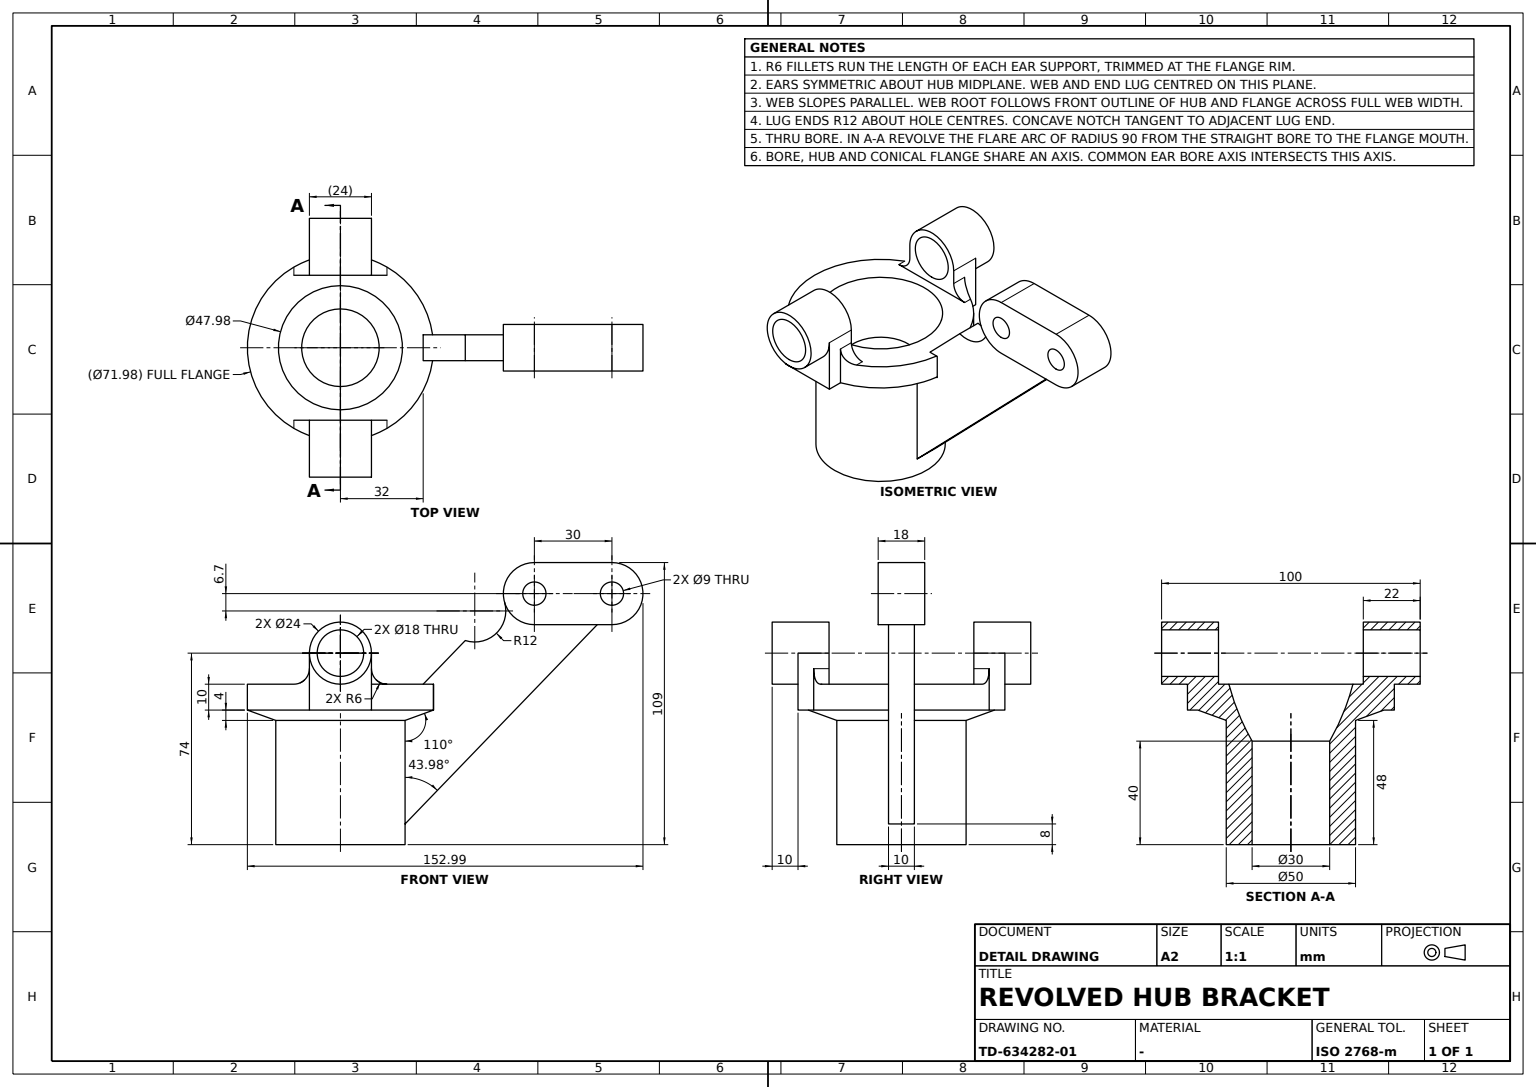
CATIA V5 part; units mm, degrees
sketch "Sketch1" plane through (0, 0, 0) normal (1, 0, 0) x (0, 1, 0)
  line L0 (-25, 0.8739) -> (-25, 48.8739)
  point P0 (-25, 48.8739)
  line L1 (-15, 0.8739) -> (-15, 40.8739)
  line L2 (-25, 0.8739) -> (-15, 0.8739)
  line L3 (-25, 48.8739) -> (-35.9899, 52.8739)
  point P1 (-35.9899, 52.8739)
  arc A0 (-23.9899, 62.8739) -> (-15, 40.8739) centre (63.0883, 85.6201) ccw
  point P2 (-23.9899, 62.8739)
  line L4 (-35.9899, 52.8739) -> (-35.9899, 62.8739)
  line L5 (-35.9899, 62.8739) -> (-23.9899, 62.8739)
  point P3 (-23.9899, 62.8739)
  dimension "distance L1 L0" = 10
  dimension "length L1" = 40
  dimension "length L0" = 48
  dimension "angle L3 L0" = 110
  dimension "radius A0" = 90
  dimension "distance P0 P1 y axis" = 4
  dimension "distance y axis L1" = 15
  dimension "length L4" = 10
  dimension "length L5" = 12
  constraint vertical L0 y-axis
  constraint vertical L1 y-axis
  constraint vertical L4 y-axis
  constraint horizontal L2 x-axis
  constraint horizontal L5 x-axis
  constraint coincidence P3 A0
  constraint coincidence P2 P3
revolve "Shaft1" add sketch "Sketch1" angle 360 about axis through (0, 0, 0) along (0, 0, 1)
ref_plane "Plane1" through (50, 0, 0) normal (1, 0, 0) x (0, 1, 0)
sketch "Sketch2" plane through (50, 0, 0) normal (1, 0, 0) x (0, 1, 0)
  circle A0 centre (0, 74.8739) radius 9
  point P0 (0, 74.8739)
  circle A1 centre (0, 74.8739) radius 12
  point P1 (0, 62.8739)
  line L0 (-25, 0.8739) -> (25, 0.8739) construction
  dimension "distance P0 L0" = 74
  dimension "radius A0" = 9
  dimension "radius A1" = 12
  constraint coincidence A1 P1
  constraint coincidence P1 y-axis
  constraint coincidence P0 y-axis
extrude "Pad1" add sketch "Sketch2" against normal blind 22
ref_plane "Plane2" through (40, 0, 0) normal (1, 0, 0) x (0, 1, 0)
sketch "Sketch3" plane through (40, 0, 0) normal (1, 0, 0) x (0, 1, 0)
  line L0 (-12, 74.8739) -> (-12, 52.8739)
  point P0 (-12, 74.8739)
  point P1 (-12, 52.8739)
  point P2 (12, 74.8739)
  point P3 (12, 52.8739)
  line L1 (12, 74.8739) -> (12, 52.8739)
  circle A0 centre (0, 74.8739) radius 12 construction
  arc A1 (-12, 74.8739) -> (12, 74.8739) centre (0, 74.8739) ccw
  line L2 (-35.9899, 52.8739) -> (35.9899, 52.8739) construction
  line L3 (-12, 52.8739) -> (12, 52.8739)
  point P4 (-12, 74.8739)
  point P5 (12, 74.8739)
  constraint vertical L0 y-axis
  constraint symmetry P0 P2 y-axis
  constraint symmetry P1 P3 y-axis
  constraint symmetry L0 L1 y-axis
  constraint tangency L0 A0
  constraint coincidence P2 A0
  constraint coincidence P1 L2
  constraint coincidence L1 P5
  constraint coincidence L0 P4
  constraint coincidence P0 P4
  constraint coincidence P2 P5
extrude "Pad2" add sketch "Sketch3" against normal up to surface (12 mm away)
fillet "Fillet1" radius 6 2 edges at (30.9652, 12, 62.8739) (30.9652, -12, 62.8739)
mirror "Mirror1" about plane through (0, 0, 0) normal (1, 0, 0) of "Pad1"
ref_plane "Plane3" through (-40, 0, 0) normal (1, 0, 0) x (0, 1, 0)
sketch "Sketch4" plane through (-40, 0, 0) normal (1, 0, 0) x (0, 1, 0)
  line L0 (12, 52.8739) -> (12, 74.8739)
  line L1 (-12, 74.8739) -> (-12, 52.8739)
  arc A0 (-12, 74.8739) -> (12, 74.8739) centre (0, 74.8739) ccw
  line L2 (-12, 52.8739) -> (12, 52.8739)
extrude "Pad3" add sketch "Sketch4" along normal up to surface (12 mm away)
fillet "Fillet2" radius 6 2 edges at (-30.9652, 12, 62.8739) (-30.9652, -12, 62.8739)
sketch "Sketch5" plane through (0, 0, 0) normal (1, 0, 0) x (0, 1, 0)
  arc A0 (63.4776, 94.5223) -> (75, 85.8739) centre (75, 97.8739) ccw
  point P0 (75, 97.8739)
  circle A1 centre (0, 74.8739) radius 12 construction
  arc A2 (48.2839, 79.7461) -> (63.4776, 94.5223) centre (51.9551, 91.1707) ccw
  point P1 (32, 62.8739)
  line L0 (-35.9899, 62.8739) -> (35.9899, 62.8739) construction
  point P2 (35.9899, 62.8739)
  line L1 (35.9899, 62.8739) -> (35.9899, 52.8739)
  point P3 (35.9899, 52.8739)
  line L2 (-35.9899, 62.8739) -> (35.9899, 62.8739) construction
  line L3 (32, 62.8739) -> (35.9899, 62.8739)
  point P4 (35.9899, 62.8739)
  line L4 (35.9899, 52.8739) -> (25, 48.8739)
  point P5 (25, 48.8739)
  point P6 (0, 39.7747)
  point P7 (35.9899, 52.8739)
  line L5 (25, 8.8739) -> (25, 48.8739)
  point P8 (25, 48.8739)
  line L6 (48.2839, 79.7461) -> (32, 62.8739)
  line L7 (25, 8.8739) -> (99.3152, 85.8739)
  point P9 (99.3152, 85.8739)
  line L8 (75, 85.8739) -> (99.3152, 85.8739)
  point P10 (99.3152, 85.8739)
  dimension "radius A0" = 12
  dimension "distance y axis P0" = 75
  dimension "distance A1 P0 y axis" = 35
  dimension "radius A2" = 12
  dimension "D5" = 32
  dimension "distance L5 y axis" = 25
  dimension "length L5" = 40
  constraint tangency A2 A0
  constraint tangency L8 A0
  constraint coincidence L0 P1
  constraint coincidence P2 L2
  constraint coincidence P2 P4
  constraint coincidence P6 L4
  constraint coincidence P7 P3
  constraint coincidence P8 P5
  constraint coincidence P9 P10
  constraint vertical L1 y-axis
  constraint vertical L5 y-axis
  constraint parallelism L7 L6
extrude "Pad4" add sketch "Sketch5" along normal mid plane 10
sketch "Sketch6" plane through (0, 0, 0) normal (1, 0, 0) x (0, 1, 0)
  arc A0 (75, 109.8739) -> (75, 85.8739) centre (75, 97.8739) ccw
  point P0 (75, 97.8739)
  arc A1 (63.4776, 94.5223) -> (75, 85.8739) centre (75, 97.8739) ccw construction
  arc A2 (105, 85.8739) -> (105, 109.8739) centre (105, 97.8739) ccw
  point P1 (105, 97.8739)
  line L0 (75, 109.8739) -> (105, 109.8739)
  line L1 (75, 85.8739) -> (105, 85.8739)
  circle A3 centre (75, 97.8739) radius 4.5
  circle A4 centre (105, 97.8739) radius 4.5
  dimension "distance P1 P0" = 30
  dimension "radius A0" = 12
  dimension "radius A4" = 4.5
  dimension "radius A3" = 4.5
  constraint concentricity A0 A1
  constraint horizontal L0 x-axis
  constraint horizontal L1 x-axis
  constraint tangency L0 A0
  constraint tangency A2 L0
  constraint tangency L1 A0
  constraint tangency L1 A2
extrude "Pad5" add sketch "Sketch6" along normal mid plane 18
